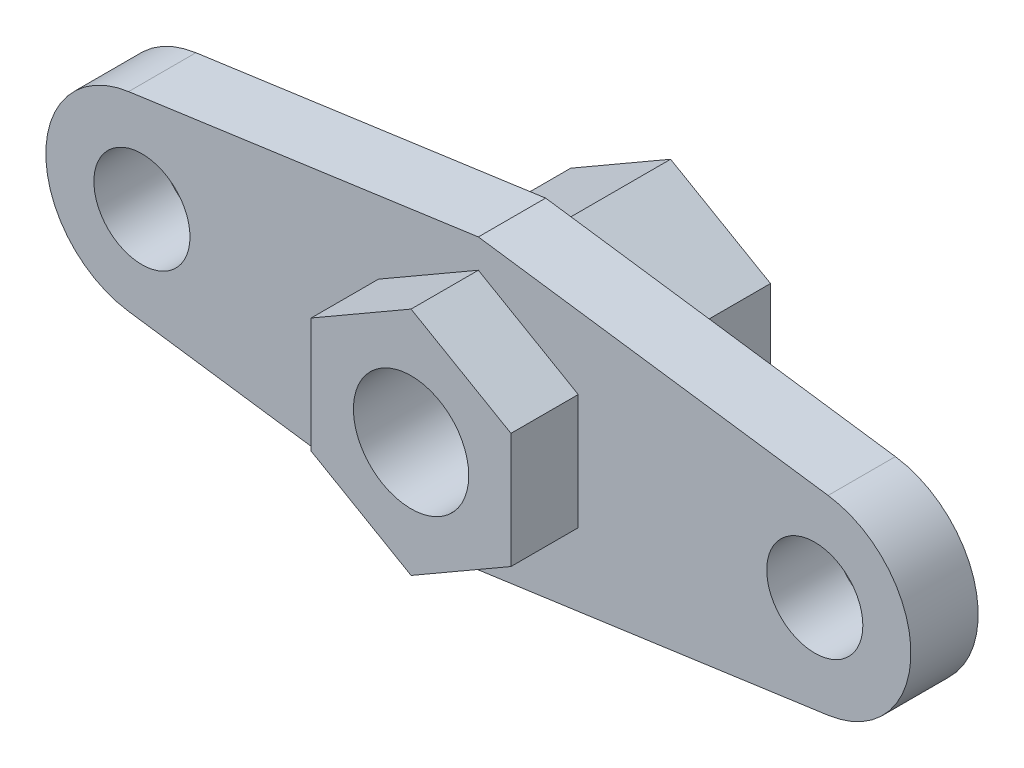
ISO-10303-21;
HEADER;
FILE_DESCRIPTION(('STEP AP214'),'2;1');
FILE_NAME('part.step','',(''),(''),'','','');
FILE_SCHEMA(('AUTOMOTIVE_DESIGN { 1 0 10303 214 1 1 1 1 }'));
ENDSEC;
DATA;
#1=APPLICATION_CONTEXT('core data for automotive mechanical design processes');
#2=APPLICATION_PROTOCOL_DEFINITION('international standard','automotive_design',2000,#1);
#3=PRODUCT_CONTEXT('',#1,'mechanical');
#4=PRODUCT('Part','Part','',(#3));
#5=PRODUCT_RELATED_PRODUCT_CATEGORY('part','',(#4));
#6=PRODUCT_DEFINITION_FORMATION('','',#4);
#7=PRODUCT_DEFINITION_CONTEXT('part definition',#1,'design');
#8=PRODUCT_DEFINITION('design','',#6,#7);
#9=PRODUCT_DEFINITION_SHAPE('','',#8);
#10=(LENGTH_UNIT() NAMED_UNIT(*) SI_UNIT(.MILLI.,.METRE.));
#11=(NAMED_UNIT(*) PLANE_ANGLE_UNIT() SI_UNIT($,.RADIAN.));
#12=(NAMED_UNIT(*) SI_UNIT($,.STERADIAN.) SOLID_ANGLE_UNIT());
#13=UNCERTAINTY_MEASURE_WITH_UNIT(LENGTH_MEASURE(1.E-05),#10,'distance_accuracy_value','');
#14=(GEOMETRIC_REPRESENTATION_CONTEXT(3) GLOBAL_UNCERTAINTY_ASSIGNED_CONTEXT((#13)) GLOBAL_UNIT_ASSIGNED_CONTEXT((#10,
#11,#12)) REPRESENTATION_CONTEXT('',''));
#15=CARTESIAN_POINT('',(0.,0.,0.));
#16=DIRECTION('',(0.,0.,1.));
#17=DIRECTION('',(1.,0.,0.));
#18=AXIS2_PLACEMENT_3D('',#15,#16,#17);
#19=CARTESIAN_POINT('',(2.43705878697643,-17.3991075068111,3.5));
#20=DIRECTION('',(0.138713925604286,-0.990332493076668,0.));
#21=DIRECTION('',(0.990332493076668,0.138713925604286,0.));
#22=AXIS2_PLACEMENT_3D('',#19,#20,#21);
#23=PLANE('',#22);
#24=DIRECTION('',(-0.990332493076668,-0.138713925604286,0.));
#25=VECTOR('',#24,1.);
#26=CARTESIAN_POINT('',(2.43705878697643,-17.3991075068111,-3.5));
#27=LINE('',#26,#25);
#28=CARTESIAN_POINT('',(55.9523566473472,-9.90332493076667,-3.5));
#29=VERTEX_POINT('',#28);
#30=CARTESIAN_POINT('',(19.5652173913043,-15.,-3.5));
#31=VERTEX_POINT('',#30);
#32=EDGE_CURVE('E156',#29,#31,#27,.T.);
#33=ORIENTED_EDGE('',*,*,#32,.F.);
#34=DIRECTION('',(0.,0.,-1.));
#35=VECTOR('',#34,1.);
#36=CARTESIAN_POINT('',(55.9523566473472,-9.90332493076667,3.5));
#37=LINE('',#36,#35);
#38=CARTESIAN_POINT('',(55.9523566473472,-9.90332493076667,3.5));
#39=VERTEX_POINT('',#38);
#40=EDGE_CURVE('E11',#39,#29,#37,.T.);
#41=ORIENTED_EDGE('',*,*,#40,.F.);
#42=DIRECTION('',(-0.990332493076668,-0.138713925604286,0.));
#43=VECTOR('',#42,1.);
#44=CARTESIAN_POINT('',(2.43705878697643,-17.3991075068111,3.5));
#45=LINE('',#44,#43);
#46=CARTESIAN_POINT('',(19.5652173913043,-15.,3.5));
#47=VERTEX_POINT('',#46);
#48=EDGE_CURVE('E160',#39,#47,#45,.T.);
#49=ORIENTED_EDGE('',*,*,#48,.T.);
#50=DIRECTION('',(0.,0.,-1.));
#51=VECTOR('',#50,1.);
#52=CARTESIAN_POINT('',(19.5652173913043,-15.,3.5));
#53=LINE('',#52,#51);
#54=EDGE_CURVE('E85',#47,#31,#53,.T.);
#55=ORIENTED_EDGE('',*,*,#54,.T.);
#56=EDGE_LOOP('',(#33,#41,#49,#55));
#57=FACE_BOUND('',#56,.T.);
#58=ADVANCED_FACE('F41',(#57),#23,.T.);
#59=CARTESIAN_POINT('',(54.5652173913044,0.,3.5));
#60=DIRECTION('',(0.,0.,-1.));
#61=DIRECTION('',(-1.,0.,0.));
#62=AXIS2_PLACEMENT_3D('',#59,#60,#61);
#63=CYLINDRICAL_SURFACE('',#62,10.);
#64=CARTESIAN_POINT('',(54.5652173913044,0.,-3.5));
#65=DIRECTION('',(0.,0.,1.));
#66=DIRECTION('',(1.,0.,0.));
#67=AXIS2_PLACEMENT_3D('',#64,#65,#66);
#68=CIRCLE('',#67,10.);
#69=CARTESIAN_POINT('',(55.9523566473472,9.90332493076669,-3.5));
#70=VERTEX_POINT('',#69);
#71=EDGE_CURVE('E188',#29,#70,#68,.T.);
#72=ORIENTED_EDGE('',*,*,#71,.T.);
#73=DIRECTION('',(0.,0.,-1.));
#74=VECTOR('',#73,1.);
#75=CARTESIAN_POINT('',(55.9523566473472,9.90332493076669,3.5));
#76=LINE('',#75,#74);
#77=CARTESIAN_POINT('',(55.9523566473472,9.90332493076669,3.5));
#78=VERTEX_POINT('',#77);
#79=EDGE_CURVE('E47',#78,#70,#76,.T.);
#80=ORIENTED_EDGE('',*,*,#79,.F.);
#81=CARTESIAN_POINT('',(54.5652173913044,0.,3.5));
#82=DIRECTION('',(0.,0.,1.));
#83=DIRECTION('',(1.,0.,0.));
#84=AXIS2_PLACEMENT_3D('',#81,#82,#83);
#85=CIRCLE('',#84,10.);
#86=EDGE_CURVE('E157',#39,#78,#85,.T.);
#87=ORIENTED_EDGE('',*,*,#86,.F.);
#88=ORIENTED_EDGE('',*,*,#40,.T.);
#89=EDGE_LOOP('',(#72,#80,#87,#88));
#90=FACE_BOUND('',#89,.T.);
#91=ADVANCED_FACE('F237',(#90),#63,.T.);
#92=CARTESIAN_POINT('',(2.43705878697642,17.3991075068111,3.5));
#93=DIRECTION('',(0.138713925604286,0.990332493076668,0.));
#94=DIRECTION('',(-0.990332493076668,0.138713925604286,0.));
#95=AXIS2_PLACEMENT_3D('',#92,#93,#94);
#96=PLANE('',#95);
#97=DIRECTION('',(0.990332493076668,-0.138713925604286,0.));
#98=VECTOR('',#97,1.);
#99=CARTESIAN_POINT('',(2.43705878697642,17.3991075068111,-3.5));
#100=LINE('',#99,#98);
#101=CARTESIAN_POINT('',(19.5652173913043,15.,-3.5));
#102=VERTEX_POINT('',#101);
#103=EDGE_CURVE('E187',#102,#70,#100,.T.);
#104=ORIENTED_EDGE('',*,*,#103,.F.);
#105=DIRECTION('',(0.,0.,-1.));
#106=VECTOR('',#105,1.);
#107=CARTESIAN_POINT('',(19.5652173913043,15.,3.5));
#108=LINE('',#107,#106);
#109=CARTESIAN_POINT('',(19.5652173913043,15.,3.5));
#110=VERTEX_POINT('',#109);
#111=EDGE_CURVE('E226',#110,#102,#108,.T.);
#112=ORIENTED_EDGE('',*,*,#111,.F.);
#113=DIRECTION('',(0.990332493076668,-0.138713925604286,0.));
#114=VECTOR('',#113,1.);
#115=CARTESIAN_POINT('',(2.43705878697642,17.3991075068111,3.5));
#116=LINE('',#115,#114);
#117=EDGE_CURVE('E165',#110,#78,#116,.T.);
#118=ORIENTED_EDGE('',*,*,#117,.T.);
#119=ORIENTED_EDGE('',*,*,#79,.T.);
#120=EDGE_LOOP('',(#104,#112,#118,#119));
#121=FACE_BOUND('',#120,.T.);
#122=ADVANCED_FACE('F231',(#121),#96,.T.);
#123=CARTESIAN_POINT('',(-1.68412844606789,12.0236458984924,3.5));
#124=DIRECTION('',(0.138713925604286,-0.990332493076668,0.));
#125=DIRECTION('',(0.990332493076668,0.138713925604286,0.));
#126=AXIS2_PLACEMENT_3D('',#123,#124,#125);
#127=PLANE('',#126);
#128=DIRECTION('',(-0.990332493076668,-0.138713925604286,0.));
#129=VECTOR('',#128,1.);
#130=CARTESIAN_POINT('',(-1.68412844606789,12.0236458984924,-3.5));
#131=LINE('',#130,#129);
#132=CARTESIAN_POINT('',(-16.8219218647385,9.90332493076668,-3.5));
#133=VERTEX_POINT('',#132);
#134=EDGE_CURVE('E191',#102,#133,#131,.T.);
#135=ORIENTED_EDGE('',*,*,#134,.T.);
#136=DIRECTION('',(0.,0.,-1.));
#137=VECTOR('',#136,1.);
#138=CARTESIAN_POINT('',(-16.8219218647385,9.90332493076668,3.5));
#139=LINE('',#138,#137);
#140=CARTESIAN_POINT('',(-16.8219218647385,9.90332493076668,3.5));
#141=VERTEX_POINT('',#140);
#142=EDGE_CURVE('E223',#141,#133,#139,.T.);
#143=ORIENTED_EDGE('',*,*,#142,.F.);
#144=DIRECTION('',(-0.990332493076668,-0.138713925604286,0.));
#145=VECTOR('',#144,1.);
#146=CARTESIAN_POINT('',(-1.68412844606789,12.0236458984924,3.5));
#147=LINE('',#146,#145);
#148=EDGE_CURVE('E164',#110,#141,#147,.T.);
#149=ORIENTED_EDGE('',*,*,#148,.F.);
#150=ORIENTED_EDGE('',*,*,#111,.T.);
#151=EDGE_LOOP('',(#135,#143,#149,#150));
#152=FACE_BOUND('',#151,.T.);
#153=ADVANCED_FACE('F244',(#152),#127,.F.);
#154=CARTESIAN_POINT('',(-15.4347826086957,0.,3.5));
#155=DIRECTION('',(0.,0.,-1.));
#156=DIRECTION('',(-1.,0.,0.));
#157=AXIS2_PLACEMENT_3D('',#154,#155,#156);
#158=CYLINDRICAL_SURFACE('',#157,10.);
#159=CARTESIAN_POINT('',(-15.4347826086957,0.,-3.5));
#160=DIRECTION('',(0.,0.,1.));
#161=DIRECTION('',(1.,0.,0.));
#162=AXIS2_PLACEMENT_3D('',#159,#160,#161);
#163=CIRCLE('',#162,10.);
#164=CARTESIAN_POINT('',(-16.8219218647385,-9.90332493076668,-3.5));
#165=VERTEX_POINT('',#164);
#166=EDGE_CURVE('E193',#133,#165,#163,.T.);
#167=ORIENTED_EDGE('',*,*,#166,.T.);
#168=DIRECTION('',(0.,0.,-1.));
#169=VECTOR('',#168,1.);
#170=CARTESIAN_POINT('',(-16.8219218647385,-9.90332493076668,3.5));
#171=LINE('',#170,#169);
#172=CARTESIAN_POINT('',(-16.8219218647385,-9.90332493076668,3.5));
#173=VERTEX_POINT('',#172);
#174=EDGE_CURVE('E225',#173,#165,#171,.T.);
#175=ORIENTED_EDGE('',*,*,#174,.F.);
#176=CARTESIAN_POINT('',(-15.4347826086957,0.,3.5));
#177=DIRECTION('',(0.,0.,1.));
#178=DIRECTION('',(1.,0.,0.));
#179=AXIS2_PLACEMENT_3D('',#176,#177,#178);
#180=CIRCLE('',#179,10.);
#181=EDGE_CURVE('E170',#141,#173,#180,.T.);
#182=ORIENTED_EDGE('',*,*,#181,.F.);
#183=ORIENTED_EDGE('',*,*,#142,.T.);
#184=EDGE_LOOP('',(#167,#175,#182,#183));
#185=FACE_BOUND('',#184,.T.);
#186=ADVANCED_FACE('F248',(#185),#158,.T.);
#187=CARTESIAN_POINT('',(-15.4347826086957,0.,3.5));
#188=DIRECTION('',(0.,0.,-1.));
#189=DIRECTION('',(-1.,0.,0.));
#190=AXIS2_PLACEMENT_3D('',#187,#188,#189);
#191=CYLINDRICAL_SURFACE('',#190,5.);
#192=CARTESIAN_POINT('',(-15.4347826086957,0.,3.5));
#193=DIRECTION('',(0.,0.,1.));
#194=DIRECTION('',(1.,0.,0.));
#195=AXIS2_PLACEMENT_3D('',#192,#193,#194);
#196=CIRCLE('',#195,5.);
#197=CARTESIAN_POINT('',(-10.4347826086957,0.,3.5));
#198=VERTEX_POINT('',#197);
#199=EDGE_CURVE('E172',#198,#198,#196,.T.);
#200=ORIENTED_EDGE('',*,*,#199,.T.);
#201=EDGE_LOOP('',(#200));
#202=FACE_BOUND('',#201,.T.);
#203=CARTESIAN_POINT('',(-15.4347826086957,0.,-3.5));
#204=DIRECTION('',(0.,0.,1.));
#205=DIRECTION('',(1.,0.,0.));
#206=AXIS2_PLACEMENT_3D('',#203,#204,#205);
#207=CIRCLE('',#206,5.);
#208=CARTESIAN_POINT('',(-10.4347826086957,0.,-3.5));
#209=VERTEX_POINT('',#208);
#210=EDGE_CURVE('E203',#209,#209,#207,.T.);
#211=ORIENTED_EDGE('',*,*,#210,.F.);
#212=EDGE_LOOP('',(#211));
#213=FACE_BOUND('',#212,.T.);
#214=ADVANCED_FACE('F268',(#202,#213),#191,.F.);
#215=CARTESIAN_POINT('',(54.5652173913044,0.,3.5));
#216=DIRECTION('',(0.,0.,-1.));
#217=DIRECTION('',(-1.,0.,0.));
#218=AXIS2_PLACEMENT_3D('',#215,#216,#217);
#219=CYLINDRICAL_SURFACE('',#218,5.);
#220=CARTESIAN_POINT('',(54.5652173913044,0.,3.5));
#221=DIRECTION('',(0.,0.,1.));
#222=DIRECTION('',(1.,0.,0.));
#223=AXIS2_PLACEMENT_3D('',#220,#221,#222);
#224=CIRCLE('',#223,5.);
#225=CARTESIAN_POINT('',(59.5652173913043,0.,3.5));
#226=VERTEX_POINT('',#225);
#227=EDGE_CURVE('E173',#226,#226,#224,.T.);
#228=ORIENTED_EDGE('',*,*,#227,.T.);
#229=EDGE_LOOP('',(#228));
#230=FACE_BOUND('',#229,.T.);
#231=CARTESIAN_POINT('',(54.5652173913044,0.,-3.5));
#232=DIRECTION('',(0.,0.,1.));
#233=DIRECTION('',(1.,0.,0.));
#234=AXIS2_PLACEMENT_3D('',#231,#232,#233);
#235=CIRCLE('',#234,5.);
#236=CARTESIAN_POINT('',(59.5652173913043,0.,-3.5));
#237=VERTEX_POINT('',#236);
#238=EDGE_CURVE('E196',#237,#237,#235,.T.);
#239=ORIENTED_EDGE('',*,*,#238,.F.);
#240=EDGE_LOOP('',(#239));
#241=FACE_BOUND('',#240,.T.);
#242=ADVANCED_FACE('F275',(#230,#241),#219,.F.);
#243=CARTESIAN_POINT('',(-1.68412844606789,-12.0236458984924,3.5));
#244=DIRECTION('',(0.138713925604286,0.990332493076668,0.));
#245=DIRECTION('',(-0.990332493076668,0.138713925604286,0.));
#246=AXIS2_PLACEMENT_3D('',#243,#244,#245);
#247=PLANE('',#246);
#248=DIRECTION('',(0.990332493076668,-0.138713925604286,0.));
#249=VECTOR('',#248,1.);
#250=CARTESIAN_POINT('',(-1.68412844606789,-12.0236458984924,-3.5));
#251=LINE('',#250,#249);
#252=EDGE_CURVE('E198',#165,#31,#251,.T.);
#253=ORIENTED_EDGE('',*,*,#252,.T.);
#254=ORIENTED_EDGE('',*,*,#54,.F.);
#255=DIRECTION('',(0.990332493076668,-0.138713925604286,0.));
#256=VECTOR('',#255,1.);
#257=CARTESIAN_POINT('',(-1.68412844606789,-12.0236458984924,3.5));
#258=LINE('',#257,#256);
#259=EDGE_CURVE('E166',#173,#47,#258,.T.);
#260=ORIENTED_EDGE('',*,*,#259,.F.);
#261=ORIENTED_EDGE('',*,*,#174,.T.);
#262=EDGE_LOOP('',(#253,#254,#260,#261));
#263=FACE_BOUND('',#262,.T.);
#264=ADVANCED_FACE('F267',(#263),#247,.F.);
#265=CARTESIAN_POINT('',(0.,0.,3.5));
#266=DIRECTION('',(0.,0.,1.));
#267=DIRECTION('',(1.,0.,0.));
#268=AXIS2_PLACEMENT_3D('',#265,#266,#267);
#269=PLANE('',#268);
#270=ORIENTED_EDGE('',*,*,#48,.F.);
#271=ORIENTED_EDGE('',*,*,#86,.T.);
#272=ORIENTED_EDGE('',*,*,#117,.F.);
#273=ORIENTED_EDGE('',*,*,#148,.T.);
#274=ORIENTED_EDGE('',*,*,#181,.T.);
#275=ORIENTED_EDGE('',*,*,#259,.T.);
#276=EDGE_LOOP('',(#270,#271,#272,#273,#274,#275));
#277=FACE_BOUND('',#276,.T.);
#278=ORIENTED_EDGE('',*,*,#227,.F.);
#279=EDGE_LOOP('',(#278));
#280=FACE_BOUND('',#279,.T.);
#281=ORIENTED_EDGE('',*,*,#199,.F.);
#282=EDGE_LOOP('',(#281));
#283=FACE_BOUND('',#282,.T.);
#284=DIRECTION('',(-0.866025403784439,0.5,0.));
#285=VECTOR('',#284,1.);
#286=CARTESIAN_POINT('',(10.0874567705327,17.4719876457173,3.5));
#287=LINE('',#286,#285);
#288=CARTESIAN_POINT('',(29.9575222367176,6.,3.5));
#289=VERTEX_POINT('',#288);
#290=CARTESIAN_POINT('',(19.5652173913044,12.,3.5));
#291=VERTEX_POINT('',#290);
#292=EDGE_CURVE('E176',#289,#291,#287,.T.);
#293=ORIENTED_EDGE('',*,*,#292,.F.);
#294=DIRECTION('',(0.,1.,0.));
#295=VECTOR('',#294,1.);
#296=CARTESIAN_POINT('',(29.9575222367176,0.,3.5));
#297=LINE('',#296,#295);
#298=CARTESIAN_POINT('',(29.9575222367176,-6.,3.5));
#299=VERTEX_POINT('',#298);
#300=EDGE_CURVE('E127',#299,#289,#297,.T.);
#301=ORIENTED_EDGE('',*,*,#300,.F.);
#302=DIRECTION('',(0.866025403784439,0.5,0.));
#303=VECTOR('',#302,1.);
#304=CARTESIAN_POINT('',(10.0874567705327,-17.4719876457173,3.5));
#305=LINE('',#304,#303);
#306=CARTESIAN_POINT('',(19.5652173913043,-12.,3.5));
#307=VERTEX_POINT('',#306);
#308=EDGE_CURVE('E124',#307,#299,#305,.T.);
#309=ORIENTED_EDGE('',*,*,#308,.F.);
#310=DIRECTION('',(0.866025403784439,-0.5,0.));
#311=VECTOR('',#310,1.);
#312=CARTESIAN_POINT('',(-0.304848074880544,-0.528012354282663,3.5));
#313=LINE('',#312,#311);
#314=CARTESIAN_POINT('',(9.17291254589109,-6.,3.5));
#315=VERTEX_POINT('',#314);
#316=EDGE_CURVE('E123',#315,#307,#313,.T.);
#317=ORIENTED_EDGE('',*,*,#316,.F.);
#318=DIRECTION('',(0.,-1.,0.));
#319=VECTOR('',#318,1.);
#320=CARTESIAN_POINT('',(9.17291254589109,0.,3.5));
#321=LINE('',#320,#319);
#322=CARTESIAN_POINT('',(9.17291254589109,6.,3.5));
#323=VERTEX_POINT('',#322);
#324=EDGE_CURVE('E60',#323,#315,#321,.T.);
#325=ORIENTED_EDGE('',*,*,#324,.F.);
#326=DIRECTION('',(-0.866025403784439,-0.5,0.));
#327=VECTOR('',#326,1.);
#328=CARTESIAN_POINT('',(-0.304848074880547,0.528012354282669,3.5));
#329=LINE('',#328,#327);
#330=EDGE_CURVE('E185',#291,#323,#329,.T.);
#331=ORIENTED_EDGE('',*,*,#330,.F.);
#332=EDGE_LOOP('',(#293,#301,#309,#317,#325,#331));
#333=FACE_BOUND('',#332,.T.);
#334=ADVANCED_FACE('F125',(#277,#280,#283,#333),#269,.T.);
#335=CARTESIAN_POINT('',(0.,0.,-3.5));
#336=DIRECTION('',(0.,0.,1.));
#337=DIRECTION('',(1.,0.,0.));
#338=AXIS2_PLACEMENT_3D('',#335,#336,#337);
#339=PLANE('',#338);
#340=ORIENTED_EDGE('',*,*,#32,.T.);
#341=ORIENTED_EDGE('',*,*,#252,.F.);
#342=ORIENTED_EDGE('',*,*,#166,.F.);
#343=ORIENTED_EDGE('',*,*,#134,.F.);
#344=ORIENTED_EDGE('',*,*,#103,.T.);
#345=ORIENTED_EDGE('',*,*,#71,.F.);
#346=EDGE_LOOP('',(#340,#341,#342,#343,#344,#345));
#347=FACE_BOUND('',#346,.T.);
#348=ORIENTED_EDGE('',*,*,#238,.T.);
#349=EDGE_LOOP('',(#348));
#350=FACE_BOUND('',#349,.T.);
#351=ORIENTED_EDGE('',*,*,#210,.T.);
#352=EDGE_LOOP('',(#351));
#353=FACE_BOUND('',#352,.T.);
#354=DIRECTION('',(-0.866025403784439,0.5,0.));
#355=VECTOR('',#354,1.);
#356=CARTESIAN_POINT('',(10.0874567705327,17.4719876457173,-3.5));
#357=LINE('',#356,#355);
#358=CARTESIAN_POINT('',(29.9575222367176,6.,-3.5));
#359=VERTEX_POINT('',#358);
#360=CARTESIAN_POINT('',(19.5652173913044,12.,-3.5));
#361=VERTEX_POINT('',#360);
#362=EDGE_CURVE('E204',#359,#361,#357,.T.);
#363=ORIENTED_EDGE('',*,*,#362,.T.);
#364=DIRECTION('',(-0.866025403784439,-0.5,0.));
#365=VECTOR('',#364,1.);
#366=CARTESIAN_POINT('',(-0.304848074880547,0.528012354282669,-3.5));
#367=LINE('',#366,#365);
#368=CARTESIAN_POINT('',(9.17291254589109,6.,-3.5));
#369=VERTEX_POINT('',#368);
#370=EDGE_CURVE('E159',#361,#369,#367,.T.);
#371=ORIENTED_EDGE('',*,*,#370,.T.);
#372=DIRECTION('',(0.,-1.,0.));
#373=VECTOR('',#372,1.);
#374=CARTESIAN_POINT('',(9.17291254589109,0.,-3.5));
#375=LINE('',#374,#373);
#376=CARTESIAN_POINT('',(9.17291254589109,-6.,-3.5));
#377=VERTEX_POINT('',#376);
#378=EDGE_CURVE('E216',#369,#377,#375,.T.);
#379=ORIENTED_EDGE('',*,*,#378,.T.);
#380=DIRECTION('',(0.866025403784439,-0.5,0.));
#381=VECTOR('',#380,1.);
#382=CARTESIAN_POINT('',(-0.304848074880544,-0.528012354282663,-3.5));
#383=LINE('',#382,#381);
#384=CARTESIAN_POINT('',(19.5652173913043,-12.,-3.5));
#385=VERTEX_POINT('',#384);
#386=EDGE_CURVE('E213',#377,#385,#383,.T.);
#387=ORIENTED_EDGE('',*,*,#386,.T.);
#388=DIRECTION('',(0.866025403784439,0.5,0.));
#389=VECTOR('',#388,1.);
#390=CARTESIAN_POINT('',(10.0874567705327,-17.4719876457173,-3.5));
#391=LINE('',#390,#389);
#392=CARTESIAN_POINT('',(29.9575222367176,-6.,-3.5));
#393=VERTEX_POINT('',#392);
#394=EDGE_CURVE('E209',#385,#393,#391,.T.);
#395=ORIENTED_EDGE('',*,*,#394,.T.);
#396=DIRECTION('',(0.,1.,0.));
#397=VECTOR('',#396,1.);
#398=CARTESIAN_POINT('',(29.9575222367176,0.,-3.5));
#399=LINE('',#398,#397);
#400=EDGE_CURVE('E210',#393,#359,#399,.T.);
#401=ORIENTED_EDGE('',*,*,#400,.T.);
#402=EDGE_LOOP('',(#363,#371,#379,#387,#395,#401));
#403=FACE_BOUND('',#402,.T.);
#404=ADVANCED_FACE('F239',(#347,#350,#353,#403),#339,.F.);
#405=CARTESIAN_POINT('',(0.,0.,10.5));
#406=DIRECTION('',(0.,0.,1.));
#407=DIRECTION('',(1.,0.,0.));
#408=AXIS2_PLACEMENT_3D('',#405,#406,#407);
#409=PLANE('',#408);
#410=CARTESIAN_POINT('',(19.5652173913044,0.,10.5));
#411=DIRECTION('',(0.,0.,1.));
#412=DIRECTION('',(1.,0.,0.));
#413=AXIS2_PLACEMENT_3D('',#410,#411,#412);
#414=CIRCLE('',#413,6.);
#415=CARTESIAN_POINT('',(25.5652173913044,0.,10.5));
#416=VERTEX_POINT('',#415);
#417=EDGE_CURVE('E347',#416,#416,#414,.T.);
#418=ORIENTED_EDGE('',*,*,#417,.F.);
#419=EDGE_LOOP('',(#418));
#420=FACE_BOUND('',#419,.T.);
#421=DIRECTION('',(-0.866025403784439,-0.5,0.));
#422=VECTOR('',#421,1.);
#423=CARTESIAN_POINT('',(19.5652173913044,12.,10.5));
#424=LINE('',#423,#422);
#425=CARTESIAN_POINT('',(19.5652173913044,12.,10.5));
#426=VERTEX_POINT('',#425);
#427=CARTESIAN_POINT('',(9.17291254589109,6.,10.5));
#428=VERTEX_POINT('',#427);
#429=EDGE_CURVE('E383',#426,#428,#424,.T.);
#430=ORIENTED_EDGE('',*,*,#429,.T.);
#431=DIRECTION('',(0.,-1.,0.));
#432=VECTOR('',#431,1.);
#433=CARTESIAN_POINT('',(9.17291254589109,6.,10.5));
#434=LINE('',#433,#432);
#435=CARTESIAN_POINT('',(9.17291254589109,-6.,10.5));
#436=VERTEX_POINT('',#435);
#437=EDGE_CURVE('E390',#428,#436,#434,.T.);
#438=ORIENTED_EDGE('',*,*,#437,.T.);
#439=DIRECTION('',(0.866025403784439,-0.5,0.));
#440=VECTOR('',#439,1.);
#441=CARTESIAN_POINT('',(9.17291254589109,-6.,10.5));
#442=LINE('',#441,#440);
#443=CARTESIAN_POINT('',(19.5652173913043,-12.,10.5));
#444=VERTEX_POINT('',#443);
#445=EDGE_CURVE('E388',#436,#444,#442,.T.);
#446=ORIENTED_EDGE('',*,*,#445,.T.);
#447=DIRECTION('',(0.866025403784439,0.5,0.));
#448=VECTOR('',#447,1.);
#449=CARTESIAN_POINT('',(19.5652173913043,-12.,10.5));
#450=LINE('',#449,#448);
#451=CARTESIAN_POINT('',(29.9575222367176,-6.,10.5));
#452=VERTEX_POINT('',#451);
#453=EDGE_CURVE('E144',#444,#452,#450,.T.);
#454=ORIENTED_EDGE('',*,*,#453,.T.);
#455=DIRECTION('',(0.,1.,0.));
#456=VECTOR('',#455,1.);
#457=CARTESIAN_POINT('',(29.9575222367176,-6.,10.5));
#458=LINE('',#457,#456);
#459=CARTESIAN_POINT('',(29.9575222367176,6.,10.5));
#460=VERTEX_POINT('',#459);
#461=EDGE_CURVE('E392',#452,#460,#458,.T.);
#462=ORIENTED_EDGE('',*,*,#461,.T.);
#463=DIRECTION('',(-0.866025403784439,0.5,0.));
#464=VECTOR('',#463,1.);
#465=CARTESIAN_POINT('',(29.9575222367176,6.,10.5));
#466=LINE('',#465,#464);
#467=EDGE_CURVE('E396',#460,#426,#466,.T.);
#468=ORIENTED_EDGE('',*,*,#467,.T.);
#469=EDGE_LOOP('',(#430,#438,#446,#454,#462,#468));
#470=FACE_BOUND('',#469,.T.);
#471=ADVANCED_FACE('F285',(#420,#470),#409,.T.);
#472=CARTESIAN_POINT('',(29.9575222367176,6.,10.5));
#473=DIRECTION('',(-0.5,-0.866025403784439,0.));
#474=DIRECTION('',(0.866025403784439,-0.5,0.));
#475=AXIS2_PLACEMENT_3D('',#472,#473,#474);
#476=PLANE('',#475);
#477=ORIENTED_EDGE('',*,*,#292,.T.);
#478=DIRECTION('',(0.,0.,-1.));
#479=VECTOR('',#478,1.);
#480=CARTESIAN_POINT('',(19.5652173913044,12.,10.5));
#481=LINE('',#480,#479);
#482=EDGE_CURVE('E397',#426,#291,#481,.T.);
#483=ORIENTED_EDGE('',*,*,#482,.F.);
#484=ORIENTED_EDGE('',*,*,#467,.F.);
#485=DIRECTION('',(0.,0.,-1.));
#486=VECTOR('',#485,1.);
#487=CARTESIAN_POINT('',(29.9575222367176,6.,10.5));
#488=LINE('',#487,#486);
#489=EDGE_CURVE('E147',#460,#289,#488,.T.);
#490=ORIENTED_EDGE('',*,*,#489,.T.);
#491=EDGE_LOOP('',(#477,#483,#484,#490));
#492=FACE_BOUND('',#491,.T.);
#493=ADVANCED_FACE('F304',(#492),#476,.F.);
#494=CARTESIAN_POINT('',(29.9575222367176,-6.,10.5));
#495=DIRECTION('',(-1.,0.,0.));
#496=DIRECTION('',(0.,-1.,0.));
#497=AXIS2_PLACEMENT_3D('',#494,#495,#496);
#498=PLANE('',#497);
#499=ORIENTED_EDGE('',*,*,#300,.T.);
#500=ORIENTED_EDGE('',*,*,#489,.F.);
#501=ORIENTED_EDGE('',*,*,#461,.F.);
#502=DIRECTION('',(0.,0.,-1.));
#503=VECTOR('',#502,1.);
#504=CARTESIAN_POINT('',(29.9575222367176,-6.,10.5));
#505=LINE('',#504,#503);
#506=EDGE_CURVE('E148',#452,#299,#505,.T.);
#507=ORIENTED_EDGE('',*,*,#506,.T.);
#508=EDGE_LOOP('',(#499,#500,#501,#507));
#509=FACE_BOUND('',#508,.T.);
#510=ADVANCED_FACE('F296',(#509),#498,.F.);
#511=CARTESIAN_POINT('',(19.5652173913043,-12.,10.5));
#512=DIRECTION('',(-0.5,0.866025403784439,0.));
#513=DIRECTION('',(-0.866025403784439,-0.5,0.));
#514=AXIS2_PLACEMENT_3D('',#511,#512,#513);
#515=PLANE('',#514);
#516=ORIENTED_EDGE('',*,*,#308,.T.);
#517=ORIENTED_EDGE('',*,*,#506,.F.);
#518=ORIENTED_EDGE('',*,*,#453,.F.);
#519=DIRECTION('',(0.,0.,-1.));
#520=VECTOR('',#519,1.);
#521=CARTESIAN_POINT('',(19.5652173913043,-12.,10.5));
#522=LINE('',#521,#520);
#523=EDGE_CURVE('E140',#444,#307,#522,.T.);
#524=ORIENTED_EDGE('',*,*,#523,.T.);
#525=EDGE_LOOP('',(#516,#517,#518,#524));
#526=FACE_BOUND('',#525,.T.);
#527=ADVANCED_FACE('F141',(#526),#515,.F.);
#528=CARTESIAN_POINT('',(9.17291254589109,-6.,10.5));
#529=DIRECTION('',(0.5,0.866025403784439,0.));
#530=DIRECTION('',(-0.866025403784439,0.5,0.));
#531=AXIS2_PLACEMENT_3D('',#528,#529,#530);
#532=PLANE('',#531);
#533=ORIENTED_EDGE('',*,*,#316,.T.);
#534=ORIENTED_EDGE('',*,*,#523,.F.);
#535=ORIENTED_EDGE('',*,*,#445,.F.);
#536=DIRECTION('',(0.,0.,-1.));
#537=VECTOR('',#536,1.);
#538=CARTESIAN_POINT('',(9.17291254589109,-6.,10.5));
#539=LINE('',#538,#537);
#540=EDGE_CURVE('E143',#436,#315,#539,.T.);
#541=ORIENTED_EDGE('',*,*,#540,.T.);
#542=EDGE_LOOP('',(#533,#534,#535,#541));
#543=FACE_BOUND('',#542,.T.);
#544=ADVANCED_FACE('F134',(#543),#532,.F.);
#545=CARTESIAN_POINT('',(9.17291254589109,6.,10.5));
#546=DIRECTION('',(1.,0.,0.));
#547=DIRECTION('',(0.,0.,-1.));
#548=AXIS2_PLACEMENT_3D('',#545,#546,#547);
#549=PLANE('',#548);
#550=ORIENTED_EDGE('',*,*,#324,.T.);
#551=ORIENTED_EDGE('',*,*,#540,.F.);
#552=ORIENTED_EDGE('',*,*,#437,.F.);
#553=DIRECTION('',(0.,0.,-1.));
#554=VECTOR('',#553,1.);
#555=CARTESIAN_POINT('',(9.17291254589109,6.,10.5));
#556=LINE('',#555,#554);
#557=EDGE_CURVE('E146',#428,#323,#556,.T.);
#558=ORIENTED_EDGE('',*,*,#557,.T.);
#559=EDGE_LOOP('',(#550,#551,#552,#558));
#560=FACE_BOUND('',#559,.T.);
#561=ADVANCED_FACE('F288',(#560),#549,.F.);
#562=CARTESIAN_POINT('',(19.5652173913044,12.,10.5));
#563=DIRECTION('',(0.5,-0.866025403784439,0.));
#564=DIRECTION('',(0.866025403784439,0.5,0.));
#565=AXIS2_PLACEMENT_3D('',#562,#563,#564);
#566=PLANE('',#565);
#567=ORIENTED_EDGE('',*,*,#330,.T.);
#568=ORIENTED_EDGE('',*,*,#557,.F.);
#569=ORIENTED_EDGE('',*,*,#429,.F.);
#570=ORIENTED_EDGE('',*,*,#482,.T.);
#571=EDGE_LOOP('',(#567,#568,#569,#570));
#572=FACE_BOUND('',#571,.T.);
#573=ADVANCED_FACE('F284',(#572),#566,.F.);
#574=CARTESIAN_POINT('',(9.17291254589109,-6.,-16.5));
#575=DIRECTION('',(1.,0.,0.));
#576=DIRECTION('',(0.,0.,-1.));
#577=AXIS2_PLACEMENT_3D('',#574,#575,#576);
#578=PLANE('',#577);
#579=DIRECTION('',(0.,0.,1.));
#580=VECTOR('',#579,1.);
#581=CARTESIAN_POINT('',(9.17291254589109,-6.,-16.5));
#582=LINE('',#581,#580);
#583=CARTESIAN_POINT('',(9.17291254589109,-6.,-16.5));
#584=VERTEX_POINT('',#583);
#585=EDGE_CURVE('E366',#584,#377,#582,.T.);
#586=ORIENTED_EDGE('',*,*,#585,.T.);
#587=ORIENTED_EDGE('',*,*,#378,.F.);
#588=DIRECTION('',(0.,0.,1.));
#589=VECTOR('',#588,1.);
#590=CARTESIAN_POINT('',(9.17291254589109,6.,-16.5));
#591=LINE('',#590,#589);
#592=CARTESIAN_POINT('',(9.17291254589109,6.,-16.5));
#593=VERTEX_POINT('',#592);
#594=EDGE_CURVE('E381',#593,#369,#591,.T.);
#595=ORIENTED_EDGE('',*,*,#594,.F.);
#596=DIRECTION('',(0.,1.,0.));
#597=VECTOR('',#596,1.);
#598=CARTESIAN_POINT('',(9.17291254589109,-6.,-16.5));
#599=LINE('',#598,#597);
#600=EDGE_CURVE('E346',#584,#593,#599,.T.);
#601=ORIENTED_EDGE('',*,*,#600,.F.);
#602=EDGE_LOOP('',(#586,#587,#595,#601));
#603=FACE_BOUND('',#602,.T.);
#604=ADVANCED_FACE('F290',(#603),#578,.F.);
#605=CARTESIAN_POINT('',(9.17291254589109,6.,-16.5));
#606=DIRECTION('',(0.5,-0.866025403784439,0.));
#607=DIRECTION('',(0.866025403784439,0.5,0.));
#608=AXIS2_PLACEMENT_3D('',#605,#606,#607);
#609=PLANE('',#608);
#610=ORIENTED_EDGE('',*,*,#594,.T.);
#611=ORIENTED_EDGE('',*,*,#370,.F.);
#612=DIRECTION('',(0.,0.,1.));
#613=VECTOR('',#612,1.);
#614=CARTESIAN_POINT('',(19.5652173913044,12.,-16.5));
#615=LINE('',#614,#613);
#616=CARTESIAN_POINT('',(19.5652173913044,12.,-16.5));
#617=VERTEX_POINT('',#616);
#618=EDGE_CURVE('E378',#617,#361,#615,.T.);
#619=ORIENTED_EDGE('',*,*,#618,.F.);
#620=DIRECTION('',(0.866025403784439,0.5,0.));
#621=VECTOR('',#620,1.);
#622=CARTESIAN_POINT('',(9.17291254589109,6.,-16.5));
#623=LINE('',#622,#621);
#624=EDGE_CURVE('E351',#593,#617,#623,.T.);
#625=ORIENTED_EDGE('',*,*,#624,.F.);
#626=EDGE_LOOP('',(#610,#611,#619,#625));
#627=FACE_BOUND('',#626,.T.);
#628=ADVANCED_FACE('F313',(#627),#609,.F.);
#629=CARTESIAN_POINT('',(19.5652173913044,12.,-16.5));
#630=DIRECTION('',(-0.5,-0.866025403784439,0.));
#631=DIRECTION('',(0.866025403784439,-0.5,0.));
#632=AXIS2_PLACEMENT_3D('',#629,#630,#631);
#633=PLANE('',#632);
#634=ORIENTED_EDGE('',*,*,#618,.T.);
#635=ORIENTED_EDGE('',*,*,#362,.F.);
#636=DIRECTION('',(0.,0.,1.));
#637=VECTOR('',#636,1.);
#638=CARTESIAN_POINT('',(29.9575222367176,6.,-16.5));
#639=LINE('',#638,#637);
#640=CARTESIAN_POINT('',(29.9575222367176,6.,-16.5));
#641=VERTEX_POINT('',#640);
#642=EDGE_CURVE('E374',#641,#359,#639,.T.);
#643=ORIENTED_EDGE('',*,*,#642,.F.);
#644=DIRECTION('',(0.866025403784439,-0.5,0.));
#645=VECTOR('',#644,1.);
#646=CARTESIAN_POINT('',(19.5652173913044,12.,-16.5));
#647=LINE('',#646,#645);
#648=EDGE_CURVE('E359',#617,#641,#647,.T.);
#649=ORIENTED_EDGE('',*,*,#648,.F.);
#650=EDGE_LOOP('',(#634,#635,#643,#649));
#651=FACE_BOUND('',#650,.T.);
#652=ADVANCED_FACE('F312',(#651),#633,.F.);
#653=CARTESIAN_POINT('',(29.9575222367176,6.,-16.5));
#654=DIRECTION('',(-1.,0.,0.));
#655=DIRECTION('',(0.,-1.,0.));
#656=AXIS2_PLACEMENT_3D('',#653,#654,#655);
#657=PLANE('',#656);
#658=ORIENTED_EDGE('',*,*,#642,.T.);
#659=ORIENTED_EDGE('',*,*,#400,.F.);
#660=DIRECTION('',(0.,0.,1.));
#661=VECTOR('',#660,1.);
#662=CARTESIAN_POINT('',(29.9575222367176,-6.,-16.5));
#663=LINE('',#662,#661);
#664=CARTESIAN_POINT('',(29.9575222367176,-6.,-16.5));
#665=VERTEX_POINT('',#664);
#666=EDGE_CURVE('E375',#665,#393,#663,.T.);
#667=ORIENTED_EDGE('',*,*,#666,.F.);
#668=DIRECTION('',(0.,-1.,0.));
#669=VECTOR('',#668,1.);
#670=CARTESIAN_POINT('',(29.9575222367176,6.,-16.5));
#671=LINE('',#670,#669);
#672=EDGE_CURVE('E358',#641,#665,#671,.T.);
#673=ORIENTED_EDGE('',*,*,#672,.F.);
#674=EDGE_LOOP('',(#658,#659,#667,#673));
#675=FACE_BOUND('',#674,.T.);
#676=ADVANCED_FACE('F317',(#675),#657,.F.);
#677=CARTESIAN_POINT('',(29.9575222367176,-6.,-16.5));
#678=DIRECTION('',(-0.5,0.866025403784439,0.));
#679=DIRECTION('',(-0.866025403784439,-0.5,0.));
#680=AXIS2_PLACEMENT_3D('',#677,#678,#679);
#681=PLANE('',#680);
#682=ORIENTED_EDGE('',*,*,#666,.T.);
#683=ORIENTED_EDGE('',*,*,#394,.F.);
#684=DIRECTION('',(0.,0.,1.));
#685=VECTOR('',#684,1.);
#686=CARTESIAN_POINT('',(19.5652173913043,-12.,-16.5));
#687=LINE('',#686,#685);
#688=CARTESIAN_POINT('',(19.5652173913043,-12.,-16.5));
#689=VERTEX_POINT('',#688);
#690=EDGE_CURVE('E93',#689,#385,#687,.T.);
#691=ORIENTED_EDGE('',*,*,#690,.F.);
#692=DIRECTION('',(-0.866025403784439,-0.5,0.));
#693=VECTOR('',#692,1.);
#694=CARTESIAN_POINT('',(29.9575222367176,-6.,-16.5));
#695=LINE('',#694,#693);
#696=EDGE_CURVE('E362',#665,#689,#695,.T.);
#697=ORIENTED_EDGE('',*,*,#696,.F.);
#698=EDGE_LOOP('',(#682,#683,#691,#697));
#699=FACE_BOUND('',#698,.T.);
#700=ADVANCED_FACE('F323',(#699),#681,.F.);
#701=CARTESIAN_POINT('',(19.5652173913043,-12.,-16.5));
#702=DIRECTION('',(0.5,0.866025403784439,0.));
#703=DIRECTION('',(-0.866025403784439,0.5,0.));
#704=AXIS2_PLACEMENT_3D('',#701,#702,#703);
#705=PLANE('',#704);
#706=ORIENTED_EDGE('',*,*,#690,.T.);
#707=ORIENTED_EDGE('',*,*,#386,.F.);
#708=ORIENTED_EDGE('',*,*,#585,.F.);
#709=DIRECTION('',(-0.866025403784439,0.5,0.));
#710=VECTOR('',#709,1.);
#711=CARTESIAN_POINT('',(19.5652173913043,-12.,-16.5));
#712=LINE('',#711,#710);
#713=EDGE_CURVE('E364',#689,#584,#712,.T.);
#714=ORIENTED_EDGE('',*,*,#713,.F.);
#715=EDGE_LOOP('',(#706,#707,#708,#714));
#716=FACE_BOUND('',#715,.T.);
#717=ADVANCED_FACE('F330',(#716),#705,.F.);
#718=CARTESIAN_POINT('',(0.,0.,-16.5));
#719=DIRECTION('',(0.,0.,-1.));
#720=DIRECTION('',(-1.,0.,0.));
#721=AXIS2_PLACEMENT_3D('',#718,#719,#720);
#722=PLANE('',#721);
#723=CARTESIAN_POINT('',(19.5652173913044,0.,-16.5));
#724=DIRECTION('',(0.,0.,1.));
#725=DIRECTION('',(1.,0.,0.));
#726=AXIS2_PLACEMENT_3D('',#723,#724,#725);
#727=CIRCLE('',#726,6.);
#728=CARTESIAN_POINT('',(25.5652173913044,0.,-16.5));
#729=VERTEX_POINT('',#728);
#730=EDGE_CURVE('E345',#729,#729,#727,.T.);
#731=ORIENTED_EDGE('',*,*,#730,.T.);
#732=EDGE_LOOP('',(#731));
#733=FACE_BOUND('',#732,.T.);
#734=ORIENTED_EDGE('',*,*,#600,.T.);
#735=ORIENTED_EDGE('',*,*,#624,.T.);
#736=ORIENTED_EDGE('',*,*,#648,.T.);
#737=ORIENTED_EDGE('',*,*,#672,.T.);
#738=ORIENTED_EDGE('',*,*,#696,.T.);
#739=ORIENTED_EDGE('',*,*,#713,.T.);
#740=EDGE_LOOP('',(#734,#735,#736,#737,#738,#739));
#741=FACE_BOUND('',#740,.T.);
#742=ADVANCED_FACE('F332',(#733,#741),#722,.T.);
#743=CARTESIAN_POINT('',(19.5652173913044,0.,-16.5));
#744=DIRECTION('',(0.,0.,1.));
#745=DIRECTION('',(1.,0.,0.));
#746=AXIS2_PLACEMENT_3D('',#743,#744,#745);
#747=CYLINDRICAL_SURFACE('',#746,6.);
#748=ORIENTED_EDGE('',*,*,#730,.F.);
#749=EDGE_LOOP('',(#748));
#750=FACE_BOUND('',#749,.T.);
#751=ORIENTED_EDGE('',*,*,#417,.T.);
#752=EDGE_LOOP('',(#751));
#753=FACE_BOUND('',#752,.T.);
#754=ADVANCED_FACE('F331',(#750,#753),#747,.F.);
#755=CLOSED_SHELL('',(#58,#91,#122,#153,#186,#214,#242,#264,#334,#404,#471,#493,#510,#527,#544,
#561,#573,#604,#628,#652,#676,#700,#717,#742,#754));
#756=MANIFOLD_SOLID_BREP('B2',#755);
#757=ADVANCED_BREP_SHAPE_REPRESENTATION('',(#18,#756),#14);
#758=SHAPE_DEFINITION_REPRESENTATION(#9,#757);
ENDSEC;
END-ISO-10303-21;
